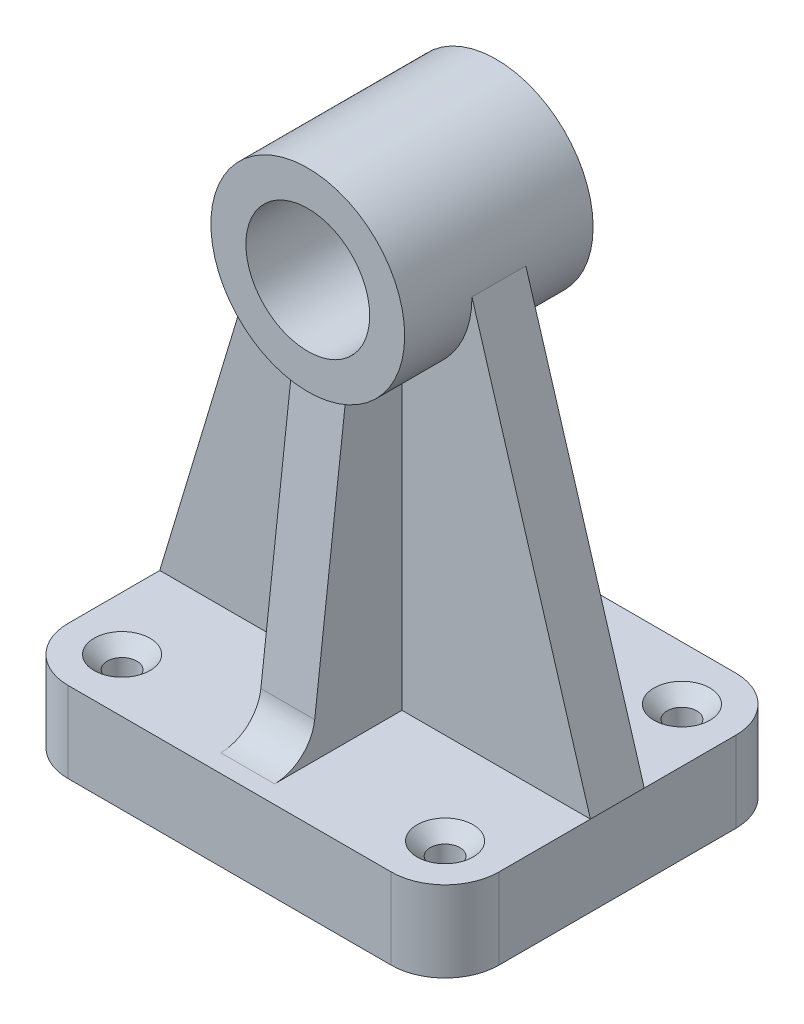
ISO-10303-21;
HEADER;
FILE_DESCRIPTION(('STEP AP214'),'2;1');
FILE_NAME('part.step','',(''),(''),'','','');
FILE_SCHEMA(('AUTOMOTIVE_DESIGN { 1 0 10303 214 1 1 1 1 }'));
ENDSEC;
DATA;
#1=APPLICATION_CONTEXT('core data for automotive mechanical design processes');
#2=APPLICATION_PROTOCOL_DEFINITION('international standard','automotive_design',2000,#1);
#3=PRODUCT_CONTEXT('',#1,'mechanical');
#4=PRODUCT('Part','Part','',(#3));
#5=PRODUCT_RELATED_PRODUCT_CATEGORY('part','',(#4));
#6=PRODUCT_DEFINITION_FORMATION('','',#4);
#7=PRODUCT_DEFINITION_CONTEXT('part definition',#1,'design');
#8=PRODUCT_DEFINITION('design','',#6,#7);
#9=PRODUCT_DEFINITION_SHAPE('','',#8);
#10=(LENGTH_UNIT() NAMED_UNIT(*) SI_UNIT(.MILLI.,.METRE.));
#11=(NAMED_UNIT(*) PLANE_ANGLE_UNIT() SI_UNIT($,.RADIAN.));
#12=(NAMED_UNIT(*) SI_UNIT($,.STERADIAN.) SOLID_ANGLE_UNIT());
#13=UNCERTAINTY_MEASURE_WITH_UNIT(LENGTH_MEASURE(1.E-05),#10,'distance_accuracy_value','');
#14=(GEOMETRIC_REPRESENTATION_CONTEXT(3) GLOBAL_UNCERTAINTY_ASSIGNED_CONTEXT((#13)) GLOBAL_UNIT_ASSIGNED_CONTEXT((#10,
#11,#12)) REPRESENTATION_CONTEXT('',''));
#15=CARTESIAN_POINT('',(0.,0.,0.));
#16=DIRECTION('',(0.,0.,1.));
#17=DIRECTION('',(1.,0.,0.));
#18=AXIS2_PLACEMENT_3D('',#15,#16,#17);
#19=CARTESIAN_POINT('',(0.,88.,5.));
#20=DIRECTION('',(0.,0.,1.));
#21=DIRECTION('',(1.,0.,0.));
#22=AXIS2_PLACEMENT_3D('',#19,#20,#21);
#23=PLANE('',#22);
#24=DIRECTION('',(1.,0.,0.));
#25=VECTOR('',#24,1.);
#26=CARTESIAN_POINT('',(-40.,15.,5.));
#27=LINE('',#26,#25);
#28=CARTESIAN_POINT('',(-40.,15.,5.));
#29=VERTEX_POINT('',#28);
#30=CARTESIAN_POINT('',(-5.,15.,5.));
#31=VERTEX_POINT('',#30);
#32=EDGE_CURVE('E209',#29,#31,#27,.T.);
#33=ORIENTED_EDGE('',*,*,#32,.T.);
#34=DIRECTION('',(0.,1.,0.));
#35=VECTOR('',#34,1.);
#36=CARTESIAN_POINT('',(-5.,88.,5.));
#37=LINE('',#36,#35);
#38=CARTESIAN_POINT('',(-5.,70.7083835342094,5.));
#39=VERTEX_POINT('',#38);
#40=EDGE_CURVE('E207',#31,#39,#37,.T.);
#41=ORIENTED_EDGE('',*,*,#40,.T.);
#42=CARTESIAN_POINT('',(0.,88.,5.));
#43=DIRECTION('',(0.,0.,-1.));
#44=DIRECTION('',(1.,0.,0.));
#45=AXIS2_PLACEMENT_3D('',#42,#43,#44);
#46=CIRCLE('',#45,18.);
#47=CARTESIAN_POINT('',(-18.,88.,5.));
#48=VERTEX_POINT('',#47);
#49=EDGE_CURVE('E195',#39,#48,#46,.T.);
#50=ORIENTED_EDGE('',*,*,#49,.T.);
#51=DIRECTION('',(-0.288550957217968,-0.95746453985962,0.));
#52=VECTOR('',#51,1.);
#53=CARTESIAN_POINT('',(-18.,88.,5.));
#54=LINE('',#53,#52);
#55=EDGE_CURVE('E305',#48,#29,#54,.T.);
#56=ORIENTED_EDGE('',*,*,#55,.T.);
#57=EDGE_LOOP('',(#33,#41,#50,#56));
#58=FACE_BOUND('',#57,.T.);
#59=ADVANCED_FACE('F44',(#58),#23,.T.);
#60=CARTESIAN_POINT('',(0.,88.,-5.));
#61=DIRECTION('',(0.,0.,1.));
#62=DIRECTION('',(1.,0.,0.));
#63=AXIS2_PLACEMENT_3D('',#60,#61,#62);
#64=PLANE('',#63);
#65=DIRECTION('',(0.,1.,0.));
#66=VECTOR('',#65,1.);
#67=CARTESIAN_POINT('',(-5.,88.,-5.));
#68=LINE('',#67,#66);
#69=CARTESIAN_POINT('',(-5.,15.,-5.));
#70=VERTEX_POINT('',#69);
#71=CARTESIAN_POINT('',(-5.,70.7083835342094,-5.));
#72=VERTEX_POINT('',#71);
#73=EDGE_CURVE('E238',#70,#72,#68,.T.);
#74=ORIENTED_EDGE('',*,*,#73,.F.);
#75=DIRECTION('',(1.,0.,0.));
#76=VECTOR('',#75,1.);
#77=CARTESIAN_POINT('',(-40.,15.,-5.));
#78=LINE('',#77,#76);
#79=CARTESIAN_POINT('',(-40.,15.,-5.));
#80=VERTEX_POINT('',#79);
#81=EDGE_CURVE('E320',#80,#70,#78,.T.);
#82=ORIENTED_EDGE('',*,*,#81,.F.);
#83=DIRECTION('',(-0.288550957217968,-0.95746453985962,0.));
#84=VECTOR('',#83,1.);
#85=CARTESIAN_POINT('',(-18.,88.,-5.));
#86=LINE('',#85,#84);
#87=CARTESIAN_POINT('',(-18.,88.,-5.));
#88=VERTEX_POINT('',#87);
#89=EDGE_CURVE('E311',#88,#80,#86,.T.);
#90=ORIENTED_EDGE('',*,*,#89,.F.);
#91=CARTESIAN_POINT('',(0.,88.,-5.));
#92=DIRECTION('',(0.,0.,-1.));
#93=DIRECTION('',(1.,0.,0.));
#94=AXIS2_PLACEMENT_3D('',#91,#92,#93);
#95=CIRCLE('',#94,18.);
#96=EDGE_CURVE('E296',#72,#88,#95,.T.);
#97=ORIENTED_EDGE('',*,*,#96,.F.);
#98=EDGE_LOOP('',(#74,#82,#90,#97));
#99=FACE_BOUND('',#98,.T.);
#100=ADVANCED_FACE('F429',(#99),#64,.F.);
#101=CARTESIAN_POINT('',(-30.,15.,22.));
#102=DIRECTION('',(0.,1.,0.));
#103=DIRECTION('',(0.,0.,1.));
#104=AXIS2_PLACEMENT_3D('',#101,#102,#103);
#105=PLANE('',#104);
#106=DIRECTION('',(-1.,0.,0.));
#107=VECTOR('',#106,1.);
#108=CARTESIAN_POINT('',(29.9999999999999,15.,-32.));
#109=LINE('',#108,#107);
#110=CARTESIAN_POINT('',(29.9999999999999,15.,-32.));
#111=VERTEX_POINT('',#110);
#112=CARTESIAN_POINT('',(-29.9999999999999,15.,-32.));
#113=VERTEX_POINT('',#112);
#114=EDGE_CURVE('E343',#111,#113,#109,.T.);
#115=ORIENTED_EDGE('',*,*,#114,.T.);
#116=CARTESIAN_POINT('',(-30.,15.,-22.));
#117=DIRECTION('',(0.,1.,0.));
#118=DIRECTION('',(0.,0.,1.));
#119=AXIS2_PLACEMENT_3D('',#116,#117,#118);
#120=CIRCLE('',#119,10.);
#121=CARTESIAN_POINT('',(-40.,15.,-21.9999999999999));
#122=VERTEX_POINT('',#121);
#123=EDGE_CURVE('E347',#113,#122,#120,.T.);
#124=ORIENTED_EDGE('',*,*,#123,.T.);
#125=DIRECTION('',(0.,0.,1.));
#126=VECTOR('',#125,1.);
#127=CARTESIAN_POINT('',(-40.,15.,-21.9999999999999));
#128=LINE('',#127,#126);
#129=EDGE_CURVE('E349',#122,#80,#128,.T.);
#130=ORIENTED_EDGE('',*,*,#129,.T.);
#131=ORIENTED_EDGE('',*,*,#81,.T.);
#132=DIRECTION('',(0.,0.,-1.));
#133=VECTOR('',#132,1.);
#134=CARTESIAN_POINT('',(-5.,15.,22.));
#135=LINE('',#134,#133);
#136=CARTESIAN_POINT('',(-5.,15.,-28.6658307795573));
#137=VERTEX_POINT('',#136);
#138=EDGE_CURVE('E245',#70,#137,#135,.T.);
#139=ORIENTED_EDGE('',*,*,#138,.T.);
#140=DIRECTION('',(1.,0.,0.));
#141=VECTOR('',#140,1.);
#142=CARTESIAN_POINT('',(5.,15.,-28.6658307795573));
#143=LINE('',#142,#141);
#144=CARTESIAN_POINT('',(5.,15.,-28.6658307795573));
#145=VERTEX_POINT('',#144);
#146=EDGE_CURVE('E393',#137,#145,#143,.T.);
#147=ORIENTED_EDGE('',*,*,#146,.T.);
#148=DIRECTION('',(0.,0.,-1.));
#149=VECTOR('',#148,1.);
#150=CARTESIAN_POINT('',(5.,15.,22.));
#151=LINE('',#150,#149);
#152=CARTESIAN_POINT('',(5.,15.,-5.));
#153=VERTEX_POINT('',#152);
#154=EDGE_CURVE('E248',#153,#145,#151,.T.);
#155=ORIENTED_EDGE('',*,*,#154,.F.);
#156=CARTESIAN_POINT('',(40.,15.,-5.));
#157=VERTEX_POINT('',#156);
#158=EDGE_CURVE('E316',#153,#157,#78,.T.);
#159=ORIENTED_EDGE('',*,*,#158,.T.);
#160=DIRECTION('',(0.,0.,-1.));
#161=VECTOR('',#160,1.);
#162=CARTESIAN_POINT('',(40.,15.,21.9999999999999));
#163=LINE('',#162,#161);
#164=CARTESIAN_POINT('',(40.,15.,-21.9999999999999));
#165=VERTEX_POINT('',#164);
#166=EDGE_CURVE('E340',#157,#165,#163,.T.);
#167=ORIENTED_EDGE('',*,*,#166,.T.);
#168=CARTESIAN_POINT('',(30.,15.,-22.));
#169=DIRECTION('',(0.,1.,0.));
#170=DIRECTION('',(0.,0.,1.));
#171=AXIS2_PLACEMENT_3D('',#168,#169,#170);
#172=CIRCLE('',#171,10.);
#173=EDGE_CURVE('E341',#165,#111,#172,.T.);
#174=ORIENTED_EDGE('',*,*,#173,.T.);
#175=EDGE_LOOP('',(#115,#124,#130,#131,#139,#147,#155,#159,#167,#174));
#176=FACE_BOUND('',#175,.T.);
#177=CARTESIAN_POINT('',(30.,15.,-22.));
#178=DIRECTION('',(0.,1.,0.));
#179=DIRECTION('',(0.,0.,1.));
#180=AXIS2_PLACEMENT_3D('',#177,#178,#179);
#181=CIRCLE('',#180,5.2);
#182=CARTESIAN_POINT('',(30.,15.,-16.8));
#183=VERTEX_POINT('',#182);
#184=EDGE_CURVE('E265',#183,#183,#181,.T.);
#185=ORIENTED_EDGE('',*,*,#184,.F.);
#186=EDGE_LOOP('',(#185));
#187=FACE_BOUND('',#186,.T.);
#188=CARTESIAN_POINT('',(-30.,15.,-22.));
#189=DIRECTION('',(0.,1.,0.));
#190=DIRECTION('',(0.,0.,1.));
#191=AXIS2_PLACEMENT_3D('',#188,#189,#190);
#192=CIRCLE('',#191,5.2);
#193=CARTESIAN_POINT('',(-30.,15.,-16.8));
#194=VERTEX_POINT('',#193);
#195=EDGE_CURVE('E251',#194,#194,#192,.T.);
#196=ORIENTED_EDGE('',*,*,#195,.F.);
#197=EDGE_LOOP('',(#196));
#198=FACE_BOUND('',#197,.T.);
#199=ADVANCED_FACE('F433',(#176,#187,#198),#105,.T.);
#200=CARTESIAN_POINT('',(-30.,15.,22.));
#201=DIRECTION('',(0.,-1.,0.));
#202=DIRECTION('',(0.,0.,-1.));
#203=AXIS2_PLACEMENT_3D('',#200,#201,#202);
#204=CYLINDRICAL_SURFACE('',#203,10.);
#205=CARTESIAN_POINT('',(-30.,0.,22.));
#206=DIRECTION('',(0.,1.,0.));
#207=DIRECTION('',(0.,0.,1.));
#208=AXIS2_PLACEMENT_3D('',#205,#206,#207);
#209=CIRCLE('',#208,10.);
#210=CARTESIAN_POINT('',(-40.,0.,21.9999999999999));
#211=VERTEX_POINT('',#210);
#212=CARTESIAN_POINT('',(-29.9999999999999,0.,32.));
#213=VERTEX_POINT('',#212);
#214=EDGE_CURVE('E328',#211,#213,#209,.T.);
#215=ORIENTED_EDGE('',*,*,#214,.T.);
#216=DIRECTION('',(0.,-1.,0.));
#217=VECTOR('',#216,1.);
#218=CARTESIAN_POINT('',(-29.9999999999999,15.,32.));
#219=LINE('',#218,#217);
#220=CARTESIAN_POINT('',(-29.9999999999999,15.,32.));
#221=VERTEX_POINT('',#220);
#222=EDGE_CURVE('E386',#221,#213,#219,.T.);
#223=ORIENTED_EDGE('',*,*,#222,.F.);
#224=CARTESIAN_POINT('',(-30.,15.,22.));
#225=DIRECTION('',(0.,1.,0.));
#226=DIRECTION('',(0.,0.,1.));
#227=AXIS2_PLACEMENT_3D('',#224,#225,#226);
#228=CIRCLE('',#227,10.);
#229=CARTESIAN_POINT('',(-40.,15.,21.9999999999999));
#230=VERTEX_POINT('',#229);
#231=EDGE_CURVE('E329',#230,#221,#228,.T.);
#232=ORIENTED_EDGE('',*,*,#231,.F.);
#233=DIRECTION('',(0.,-1.,0.));
#234=VECTOR('',#233,1.);
#235=CARTESIAN_POINT('',(-40.,15.,21.9999999999999));
#236=LINE('',#235,#234);
#237=EDGE_CURVE('E354',#230,#211,#236,.T.);
#238=ORIENTED_EDGE('',*,*,#237,.T.);
#239=EDGE_LOOP('',(#215,#223,#232,#238));
#240=FACE_BOUND('',#239,.T.);
#241=ADVANCED_FACE('F710',(#240),#204,.T.);
#242=CARTESIAN_POINT('',(-29.9999999999999,15.,32.));
#243=DIRECTION('',(0.,0.,-1.));
#244=DIRECTION('',(-1.,0.,0.));
#245=AXIS2_PLACEMENT_3D('',#242,#243,#244);
#246=PLANE('',#245);
#247=DIRECTION('',(0.,-1.,0.));
#248=VECTOR('',#247,1.);
#249=CARTESIAN_POINT('',(29.9999999999999,15.,32.));
#250=LINE('',#249,#248);
#251=CARTESIAN_POINT('',(29.9999999999999,15.,32.));
#252=VERTEX_POINT('',#251);
#253=CARTESIAN_POINT('',(29.9999999999999,0.,32.));
#254=VERTEX_POINT('',#253);
#255=EDGE_CURVE('E387',#252,#254,#250,.T.);
#256=ORIENTED_EDGE('',*,*,#255,.F.);
#257=DIRECTION('',(1.,0.,0.));
#258=VECTOR('',#257,1.);
#259=CARTESIAN_POINT('',(-29.9999999999999,15.,32.));
#260=LINE('',#259,#258);
#261=EDGE_CURVE('E334',#221,#252,#260,.T.);
#262=ORIENTED_EDGE('',*,*,#261,.F.);
#263=ORIENTED_EDGE('',*,*,#222,.T.);
#264=DIRECTION('',(1.,0.,0.));
#265=VECTOR('',#264,1.);
#266=CARTESIAN_POINT('',(-29.9999999999999,0.,32.));
#267=LINE('',#266,#265);
#268=EDGE_CURVE('E353',#213,#254,#267,.T.);
#269=ORIENTED_EDGE('',*,*,#268,.T.);
#270=EDGE_LOOP('',(#256,#262,#263,#269));
#271=FACE_BOUND('',#270,.T.);
#272=ADVANCED_FACE('F772',(#271),#246,.F.);
#273=CARTESIAN_POINT('',(30.,15.,22.));
#274=DIRECTION('',(0.,-1.,0.));
#275=DIRECTION('',(0.,0.,-1.));
#276=AXIS2_PLACEMENT_3D('',#273,#274,#275);
#277=CYLINDRICAL_SURFACE('',#276,10.);
#278=CARTESIAN_POINT('',(30.,0.,22.));
#279=DIRECTION('',(0.,1.,0.));
#280=DIRECTION('',(0.,0.,1.));
#281=AXIS2_PLACEMENT_3D('',#278,#279,#280);
#282=CIRCLE('',#281,10.);
#283=CARTESIAN_POINT('',(40.,0.,21.9999999999999));
#284=VERTEX_POINT('',#283);
#285=EDGE_CURVE('E356',#254,#284,#282,.T.);
#286=ORIENTED_EDGE('',*,*,#285,.T.);
#287=DIRECTION('',(0.,-1.,0.));
#288=VECTOR('',#287,1.);
#289=CARTESIAN_POINT('',(40.,15.,21.9999999999999));
#290=LINE('',#289,#288);
#291=CARTESIAN_POINT('',(40.,15.,21.9999999999999));
#292=VERTEX_POINT('',#291);
#293=EDGE_CURVE('E382',#292,#284,#290,.T.);
#294=ORIENTED_EDGE('',*,*,#293,.F.);
#295=CARTESIAN_POINT('',(30.,15.,22.));
#296=DIRECTION('',(0.,1.,0.));
#297=DIRECTION('',(0.,0.,1.));
#298=AXIS2_PLACEMENT_3D('',#295,#296,#297);
#299=CIRCLE('',#298,10.);
#300=EDGE_CURVE('E337',#252,#292,#299,.T.);
#301=ORIENTED_EDGE('',*,*,#300,.F.);
#302=ORIENTED_EDGE('',*,*,#255,.T.);
#303=EDGE_LOOP('',(#286,#294,#301,#302));
#304=FACE_BOUND('',#303,.T.);
#305=ADVANCED_FACE('F763',(#304),#277,.T.);
#306=CARTESIAN_POINT('',(40.,15.,0.));
#307=DIRECTION('',(-1.,0.,0.));
#308=DIRECTION('',(0.,0.,1.));
#309=AXIS2_PLACEMENT_3D('',#306,#307,#308);
#310=PLANE('',#309);
#311=DIRECTION('',(0.,0.,-1.));
#312=VECTOR('',#311,1.);
#313=CARTESIAN_POINT('',(40.,0.,0.));
#314=LINE('',#313,#312);
#315=CARTESIAN_POINT('',(40.,0.,-21.9999999999999));
#316=VERTEX_POINT('',#315);
#317=EDGE_CURVE('E357',#284,#316,#314,.T.);
#318=ORIENTED_EDGE('',*,*,#317,.T.);
#319=DIRECTION('',(0.,-1.,0.));
#320=VECTOR('',#319,1.);
#321=CARTESIAN_POINT('',(40.,15.,-21.9999999999999));
#322=LINE('',#321,#320);
#323=EDGE_CURVE('E379',#165,#316,#322,.T.);
#324=ORIENTED_EDGE('',*,*,#323,.F.);
#325=ORIENTED_EDGE('',*,*,#166,.F.);
#326=DIRECTION('',(0.,0.,-1.));
#327=VECTOR('',#326,1.);
#328=CARTESIAN_POINT('',(40.,15.,5.));
#329=LINE('',#328,#327);
#330=CARTESIAN_POINT('',(40.,15.,5.));
#331=VERTEX_POINT('',#330);
#332=EDGE_CURVE('E323',#331,#157,#329,.T.);
#333=ORIENTED_EDGE('',*,*,#332,.F.);
#334=EDGE_CURVE('E336',#292,#331,#163,.T.);
#335=ORIENTED_EDGE('',*,*,#334,.F.);
#336=ORIENTED_EDGE('',*,*,#293,.T.);
#337=EDGE_LOOP('',(#318,#324,#325,#333,#335,#336));
#338=FACE_BOUND('',#337,.T.);
#339=ADVANCED_FACE('F496',(#338),#310,.F.);
#340=CARTESIAN_POINT('',(30.,15.,-22.));
#341=DIRECTION('',(0.,-1.,0.));
#342=DIRECTION('',(0.,0.,-1.));
#343=AXIS2_PLACEMENT_3D('',#340,#341,#342);
#344=CYLINDRICAL_SURFACE('',#343,10.);
#345=CARTESIAN_POINT('',(30.,0.,-22.));
#346=DIRECTION('',(0.,1.,0.));
#347=DIRECTION('',(0.,0.,1.));
#348=AXIS2_PLACEMENT_3D('',#345,#346,#347);
#349=CIRCLE('',#348,10.);
#350=CARTESIAN_POINT('',(29.9999999999999,0.,-32.));
#351=VERTEX_POINT('',#350);
#352=EDGE_CURVE('E362',#316,#351,#349,.T.);
#353=ORIENTED_EDGE('',*,*,#352,.T.);
#354=DIRECTION('',(0.,-1.,0.));
#355=VECTOR('',#354,1.);
#356=CARTESIAN_POINT('',(29.9999999999999,15.,-32.));
#357=LINE('',#356,#355);
#358=EDGE_CURVE('E380',#111,#351,#357,.T.);
#359=ORIENTED_EDGE('',*,*,#358,.F.);
#360=ORIENTED_EDGE('',*,*,#173,.F.);
#361=ORIENTED_EDGE('',*,*,#323,.T.);
#362=EDGE_LOOP('',(#353,#359,#360,#361));
#363=FACE_BOUND('',#362,.T.);
#364=ADVANCED_FACE('F742',(#363),#344,.T.);
#365=CARTESIAN_POINT('',(29.9999999999999,15.,-32.));
#366=DIRECTION('',(0.,0.,1.));
#367=DIRECTION('',(1.,0.,0.));
#368=AXIS2_PLACEMENT_3D('',#365,#366,#367);
#369=PLANE('',#368);
#370=DIRECTION('',(-1.,0.,0.));
#371=VECTOR('',#370,1.);
#372=CARTESIAN_POINT('',(29.9999999999999,0.,-32.));
#373=LINE('',#372,#371);
#374=CARTESIAN_POINT('',(-29.9999999999999,0.,-32.));
#375=VERTEX_POINT('',#374);
#376=EDGE_CURVE('E365',#351,#375,#373,.T.);
#377=ORIENTED_EDGE('',*,*,#376,.T.);
#378=DIRECTION('',(0.,-1.,0.));
#379=VECTOR('',#378,1.);
#380=CARTESIAN_POINT('',(-29.9999999999999,15.,-32.));
#381=LINE('',#380,#379);
#382=EDGE_CURVE('E372',#113,#375,#381,.T.);
#383=ORIENTED_EDGE('',*,*,#382,.F.);
#384=ORIENTED_EDGE('',*,*,#114,.F.);
#385=ORIENTED_EDGE('',*,*,#358,.T.);
#386=EDGE_LOOP('',(#377,#383,#384,#385));
#387=FACE_BOUND('',#386,.T.);
#388=ADVANCED_FACE('F737',(#387),#369,.F.);
#389=CARTESIAN_POINT('',(-30.,15.,-22.));
#390=DIRECTION('',(0.,-1.,0.));
#391=DIRECTION('',(0.,0.,-1.));
#392=AXIS2_PLACEMENT_3D('',#389,#390,#391);
#393=CYLINDRICAL_SURFACE('',#392,10.);
#394=CARTESIAN_POINT('',(-30.,0.,-22.));
#395=DIRECTION('',(0.,1.,0.));
#396=DIRECTION('',(0.,0.,1.));
#397=AXIS2_PLACEMENT_3D('',#394,#395,#396);
#398=CIRCLE('',#397,10.);
#399=CARTESIAN_POINT('',(-40.,0.,-21.9999999999999));
#400=VERTEX_POINT('',#399);
#401=EDGE_CURVE('E368',#375,#400,#398,.T.);
#402=ORIENTED_EDGE('',*,*,#401,.T.);
#403=DIRECTION('',(0.,-1.,0.));
#404=VECTOR('',#403,1.);
#405=CARTESIAN_POINT('',(-40.,15.,-21.9999999999999));
#406=LINE('',#405,#404);
#407=EDGE_CURVE('E371',#122,#400,#406,.T.);
#408=ORIENTED_EDGE('',*,*,#407,.F.);
#409=ORIENTED_EDGE('',*,*,#123,.F.);
#410=ORIENTED_EDGE('',*,*,#382,.T.);
#411=EDGE_LOOP('',(#402,#408,#409,#410));
#412=FACE_BOUND('',#411,.T.);
#413=ADVANCED_FACE('F730',(#412),#393,.T.);
#414=CARTESIAN_POINT('',(-40.,15.,-21.9999999999999));
#415=DIRECTION('',(1.,0.,0.));
#416=DIRECTION('',(0.,0.,-1.));
#417=AXIS2_PLACEMENT_3D('',#414,#415,#416);
#418=PLANE('',#417);
#419=DIRECTION('',(0.,0.,1.));
#420=VECTOR('',#419,1.);
#421=CARTESIAN_POINT('',(-40.,0.,-21.9999999999999));
#422=LINE('',#421,#420);
#423=EDGE_CURVE('E331',#400,#211,#422,.T.);
#424=ORIENTED_EDGE('',*,*,#423,.T.);
#425=ORIENTED_EDGE('',*,*,#237,.F.);
#426=EDGE_CURVE('E346',#29,#230,#128,.T.);
#427=ORIENTED_EDGE('',*,*,#426,.F.);
#428=DIRECTION('',(0.,0.,-1.));
#429=VECTOR('',#428,1.);
#430=CARTESIAN_POINT('',(-40.,15.,5.));
#431=LINE('',#430,#429);
#432=EDGE_CURVE('E326',#29,#80,#431,.T.);
#433=ORIENTED_EDGE('',*,*,#432,.T.);
#434=ORIENTED_EDGE('',*,*,#129,.F.);
#435=ORIENTED_EDGE('',*,*,#407,.T.);
#436=EDGE_LOOP('',(#424,#425,#427,#433,#434,#435));
#437=FACE_BOUND('',#436,.T.);
#438=ADVANCED_FACE('F419',(#437),#418,.F.);
#439=DIRECTION('',(0.,0.,-1.));
#440=VECTOR('',#439,1.);
#441=CARTESIAN_POINT('',(5.,15.,22.));
#442=LINE('',#441,#440);
#443=CARTESIAN_POINT('',(5.,15.,28.6658307795573));
#444=VERTEX_POINT('',#443);
#445=CARTESIAN_POINT('',(5.,15.,5.));
#446=VERTEX_POINT('',#445);
#447=EDGE_CURVE('E58',#444,#446,#442,.T.);
#448=ORIENTED_EDGE('',*,*,#447,.F.);
#449=DIRECTION('',(1.,0.,0.));
#450=VECTOR('',#449,1.);
#451=CARTESIAN_POINT('',(-5.,15.,28.6658307795573));
#452=LINE('',#451,#450);
#453=CARTESIAN_POINT('',(-5.,15.,28.6658307795573));
#454=VERTEX_POINT('',#453);
#455=EDGE_CURVE('E407',#444,#454,#452,.F.);
#456=ORIENTED_EDGE('',*,*,#455,.T.);
#457=DIRECTION('',(0.,0.,-1.));
#458=VECTOR('',#457,1.);
#459=CARTESIAN_POINT('',(-5.,15.,22.));
#460=LINE('',#459,#458);
#461=EDGE_CURVE('E66',#454,#31,#460,.T.);
#462=ORIENTED_EDGE('',*,*,#461,.T.);
#463=ORIENTED_EDGE('',*,*,#32,.F.);
#464=ORIENTED_EDGE('',*,*,#426,.T.);
#465=ORIENTED_EDGE('',*,*,#231,.T.);
#466=ORIENTED_EDGE('',*,*,#261,.T.);
#467=ORIENTED_EDGE('',*,*,#300,.T.);
#468=ORIENTED_EDGE('',*,*,#334,.T.);
#469=EDGE_CURVE('E302',#446,#331,#27,.T.);
#470=ORIENTED_EDGE('',*,*,#469,.F.);
#471=EDGE_LOOP('',(#448,#456,#462,#463,#464,#465,#466,#467,#468,#470));
#472=FACE_BOUND('',#471,.T.);
#473=CARTESIAN_POINT('',(30.,15.,22.));
#474=DIRECTION('',(0.,1.,0.));
#475=DIRECTION('',(0.,0.,1.));
#476=AXIS2_PLACEMENT_3D('',#473,#474,#475);
#477=CIRCLE('',#476,5.2);
#478=CARTESIAN_POINT('',(30.,15.,27.2));
#479=VERTEX_POINT('',#478);
#480=EDGE_CURVE('E271',#479,#479,#477,.T.);
#481=ORIENTED_EDGE('',*,*,#480,.F.);
#482=EDGE_LOOP('',(#481));
#483=FACE_BOUND('',#482,.T.);
#484=CARTESIAN_POINT('',(-30.,15.,22.));
#485=DIRECTION('',(0.,1.,0.));
#486=DIRECTION('',(0.,0.,1.));
#487=AXIS2_PLACEMENT_3D('',#484,#485,#486);
#488=CIRCLE('',#487,5.2);
#489=CARTESIAN_POINT('',(-30.,15.,27.2));
#490=VERTEX_POINT('',#489);
#491=EDGE_CURVE('E278',#490,#490,#488,.T.);
#492=ORIENTED_EDGE('',*,*,#491,.F.);
#493=EDGE_LOOP('',(#492));
#494=FACE_BOUND('',#493,.T.);
#495=ADVANCED_FACE('F412',(#472,#483,#494),#105,.T.);
#496=CARTESIAN_POINT('',(-30.,0.,22.));
#497=DIRECTION('',(0.,1.,0.));
#498=DIRECTION('',(0.,0.,1.));
#499=AXIS2_PLACEMENT_3D('',#496,#497,#498);
#500=PLANE('',#499);
#501=ORIENTED_EDGE('',*,*,#401,.F.);
#502=ORIENTED_EDGE('',*,*,#376,.F.);
#503=ORIENTED_EDGE('',*,*,#352,.F.);
#504=ORIENTED_EDGE('',*,*,#317,.F.);
#505=ORIENTED_EDGE('',*,*,#285,.F.);
#506=ORIENTED_EDGE('',*,*,#268,.F.);
#507=ORIENTED_EDGE('',*,*,#214,.F.);
#508=ORIENTED_EDGE('',*,*,#423,.F.);
#509=EDGE_LOOP('',(#501,#502,#503,#504,#505,#506,#507,#508));
#510=FACE_BOUND('',#509,.T.);
#511=CARTESIAN_POINT('',(-30.,0.,-22.));
#512=DIRECTION('',(0.,1.,0.));
#513=DIRECTION('',(0.,0.,1.));
#514=AXIS2_PLACEMENT_3D('',#511,#512,#513);
#515=CIRCLE('',#514,2.75);
#516=CARTESIAN_POINT('',(-30.,0.,-19.25));
#517=VERTEX_POINT('',#516);
#518=EDGE_CURVE('E259',#517,#517,#515,.T.);
#519=ORIENTED_EDGE('',*,*,#518,.T.);
#520=EDGE_LOOP('',(#519));
#521=FACE_BOUND('',#520,.T.);
#522=CARTESIAN_POINT('',(30.,0.,-22.));
#523=DIRECTION('',(0.,1.,0.));
#524=DIRECTION('',(0.,0.,1.));
#525=AXIS2_PLACEMENT_3D('',#522,#523,#524);
#526=CIRCLE('',#525,2.75);
#527=CARTESIAN_POINT('',(30.,0.,-19.25));
#528=VERTEX_POINT('',#527);
#529=EDGE_CURVE('E268',#528,#528,#526,.T.);
#530=ORIENTED_EDGE('',*,*,#529,.T.);
#531=EDGE_LOOP('',(#530));
#532=FACE_BOUND('',#531,.T.);
#533=CARTESIAN_POINT('',(30.,0.,22.));
#534=DIRECTION('',(0.,1.,0.));
#535=DIRECTION('',(0.,0.,1.));
#536=AXIS2_PLACEMENT_3D('',#533,#534,#535);
#537=CIRCLE('',#536,2.75);
#538=CARTESIAN_POINT('',(30.,0.,24.75));
#539=VERTEX_POINT('',#538);
#540=EDGE_CURVE('E280',#539,#539,#537,.T.);
#541=ORIENTED_EDGE('',*,*,#540,.T.);
#542=EDGE_LOOP('',(#541));
#543=FACE_BOUND('',#542,.T.);
#544=CARTESIAN_POINT('',(-30.,0.,22.));
#545=DIRECTION('',(0.,1.,0.));
#546=DIRECTION('',(0.,0.,1.));
#547=AXIS2_PLACEMENT_3D('',#544,#545,#546);
#548=CIRCLE('',#547,2.75);
#549=CARTESIAN_POINT('',(-30.,0.,24.75));
#550=VERTEX_POINT('',#549);
#551=EDGE_CURVE('E289',#550,#550,#548,.T.);
#552=ORIENTED_EDGE('',*,*,#551,.T.);
#553=EDGE_LOOP('',(#552));
#554=FACE_BOUND('',#553,.T.);
#555=ADVANCED_FACE('F663',(#510,#521,#532,#543,#554),#500,.F.);
#556=CARTESIAN_POINT('',(-18.,88.,5.));
#557=DIRECTION('',(0.95746453985962,-0.288550957217968,0.));
#558=DIRECTION('',(0.288550957217968,0.95746453985962,0.));
#559=AXIS2_PLACEMENT_3D('',#556,#557,#558);
#560=PLANE('',#559);
#561=ORIENTED_EDGE('',*,*,#89,.T.);
#562=ORIENTED_EDGE('',*,*,#432,.F.);
#563=ORIENTED_EDGE('',*,*,#55,.F.);
#564=DIRECTION('',(0.,0.,-1.));
#565=VECTOR('',#564,1.);
#566=CARTESIAN_POINT('',(-18.,88.,5.));
#567=LINE('',#566,#565);
#568=EDGE_CURVE('E203',#48,#88,#567,.T.);
#569=ORIENTED_EDGE('',*,*,#568,.T.);
#570=EDGE_LOOP('',(#561,#562,#563,#569));
#571=FACE_BOUND('',#570,.T.);
#572=ADVANCED_FACE('F422',(#571),#560,.F.);
#573=CARTESIAN_POINT('',(18.,88.,5.));
#574=DIRECTION('',(-0.95746453985962,-0.288550957217968,0.));
#575=DIRECTION('',(0.288550957217968,-0.95746453985962,0.));
#576=AXIS2_PLACEMENT_3D('',#573,#574,#575);
#577=PLANE('',#576);
#578=DIRECTION('',(-0.288550957217968,0.95746453985962,0.));
#579=VECTOR('',#578,1.);
#580=CARTESIAN_POINT('',(18.,88.,-5.));
#581=LINE('',#580,#579);
#582=CARTESIAN_POINT('',(18.,88.,-5.));
#583=VERTEX_POINT('',#582);
#584=EDGE_CURVE('E206',#157,#583,#581,.T.);
#585=ORIENTED_EDGE('',*,*,#584,.T.);
#586=DIRECTION('',(0.,0.,-1.));
#587=VECTOR('',#586,1.);
#588=CARTESIAN_POINT('',(18.,88.,5.));
#589=LINE('',#588,#587);
#590=CARTESIAN_POINT('',(18.,88.,5.));
#591=VERTEX_POINT('',#590);
#592=EDGE_CURVE('E310',#591,#583,#589,.T.);
#593=ORIENTED_EDGE('',*,*,#592,.F.);
#594=DIRECTION('',(-0.288550957217968,0.95746453985962,0.));
#595=VECTOR('',#594,1.);
#596=CARTESIAN_POINT('',(18.,88.,5.));
#597=LINE('',#596,#595);
#598=EDGE_CURVE('E307',#331,#591,#597,.T.);
#599=ORIENTED_EDGE('',*,*,#598,.F.);
#600=ORIENTED_EDGE('',*,*,#332,.T.);
#601=EDGE_LOOP('',(#585,#593,#599,#600));
#602=FACE_BOUND('',#601,.T.);
#603=ADVANCED_FACE('F481',(#602),#577,.F.);
#604=DIRECTION('',(0.,1.,0.));
#605=VECTOR('',#604,1.);
#606=CARTESIAN_POINT('',(5.,88.,5.));
#607=LINE('',#606,#605);
#608=CARTESIAN_POINT('',(5.,70.7083835342094,5.));
#609=VERTEX_POINT('',#608);
#610=EDGE_CURVE('E223',#446,#609,#607,.T.);
#611=ORIENTED_EDGE('',*,*,#610,.F.);
#612=ORIENTED_EDGE('',*,*,#469,.T.);
#613=ORIENTED_EDGE('',*,*,#598,.T.);
#614=EDGE_CURVE('E202',#591,#609,#46,.T.);
#615=ORIENTED_EDGE('',*,*,#614,.T.);
#616=EDGE_LOOP('',(#611,#612,#613,#615));
#617=FACE_BOUND('',#616,.T.);
#618=ADVANCED_FACE('F472',(#617),#23,.T.);
#619=ORIENTED_EDGE('',*,*,#158,.F.);
#620=DIRECTION('',(0.,1.,0.));
#621=VECTOR('',#620,1.);
#622=CARTESIAN_POINT('',(5.,88.,-5.));
#623=LINE('',#622,#621);
#624=CARTESIAN_POINT('',(5.,70.7083835342094,-5.));
#625=VERTEX_POINT('',#624);
#626=EDGE_CURVE('E246',#153,#625,#623,.T.);
#627=ORIENTED_EDGE('',*,*,#626,.T.);
#628=EDGE_CURVE('E309',#583,#625,#95,.T.);
#629=ORIENTED_EDGE('',*,*,#628,.F.);
#630=ORIENTED_EDGE('',*,*,#584,.F.);
#631=EDGE_LOOP('',(#619,#627,#629,#630));
#632=FACE_BOUND('',#631,.T.);
#633=ADVANCED_FACE('F446',(#632),#64,.F.);
#634=CARTESIAN_POINT('',(0.,88.,17.5));
#635=DIRECTION('',(0.,0.,1.));
#636=DIRECTION('',(1.,0.,0.));
#637=AXIS2_PLACEMENT_3D('',#634,#635,#636);
#638=PLANE('',#637);
#639=CARTESIAN_POINT('',(0.,88.,17.5));
#640=DIRECTION('',(0.,0.,1.));
#641=DIRECTION('',(1.,0.,0.));
#642=AXIS2_PLACEMENT_3D('',#639,#640,#641);
#643=CIRCLE('',#642,11.5);
#644=CARTESIAN_POINT('',(11.5,88.,17.5));
#645=VERTEX_POINT('',#644);
#646=EDGE_CURVE('E287',#645,#645,#643,.T.);
#647=ORIENTED_EDGE('',*,*,#646,.F.);
#648=EDGE_LOOP('',(#647));
#649=FACE_BOUND('',#648,.T.);
#650=CARTESIAN_POINT('',(0.,88.,17.5));
#651=DIRECTION('',(0.,0.,1.));
#652=DIRECTION('',(1.,0.,0.));
#653=AXIS2_PLACEMENT_3D('',#650,#651,#652);
#654=CIRCLE('',#653,18.);
#655=CARTESIAN_POINT('',(18.,88.,17.5));
#656=VERTEX_POINT('',#655);
#657=EDGE_CURVE('E297',#656,#656,#654,.T.);
#658=ORIENTED_EDGE('',*,*,#657,.T.);
#659=EDGE_LOOP('',(#658));
#660=FACE_BOUND('',#659,.T.);
#661=ADVANCED_FACE('F488',(#649,#660),#638,.T.);
#662=CARTESIAN_POINT('',(0.,88.,-17.5));
#663=DIRECTION('',(0.,0.,1.));
#664=DIRECTION('',(1.,0.,0.));
#665=AXIS2_PLACEMENT_3D('',#662,#663,#664);
#666=PLANE('',#665);
#667=CARTESIAN_POINT('',(0.,88.,-17.5));
#668=DIRECTION('',(0.,0.,1.));
#669=DIRECTION('',(1.,0.,0.));
#670=AXIS2_PLACEMENT_3D('',#667,#668,#669);
#671=CIRCLE('',#670,11.5);
#672=CARTESIAN_POINT('',(11.5,88.,-17.5));
#673=VERTEX_POINT('',#672);
#674=EDGE_CURVE('E288',#673,#673,#671,.T.);
#675=ORIENTED_EDGE('',*,*,#674,.T.);
#676=EDGE_LOOP('',(#675));
#677=FACE_BOUND('',#676,.T.);
#678=CARTESIAN_POINT('',(0.,88.,-17.5));
#679=DIRECTION('',(0.,0.,1.));
#680=DIRECTION('',(1.,0.,0.));
#681=AXIS2_PLACEMENT_3D('',#678,#679,#680);
#682=CIRCLE('',#681,18.);
#683=CARTESIAN_POINT('',(18.,88.,-17.5));
#684=VERTEX_POINT('',#683);
#685=EDGE_CURVE('E291',#684,#684,#682,.T.);
#686=ORIENTED_EDGE('',*,*,#685,.F.);
#687=EDGE_LOOP('',(#686));
#688=FACE_BOUND('',#687,.T.);
#689=ADVANCED_FACE('F685',(#677,#688),#666,.F.);
#690=CARTESIAN_POINT('',(0.,88.,17.5));
#691=DIRECTION('',(0.,0.,-1.));
#692=DIRECTION('',(-1.,0.,0.));
#693=AXIS2_PLACEMENT_3D('',#690,#691,#692);
#694=CYLINDRICAL_SURFACE('',#693,18.);
#695=ORIENTED_EDGE('',*,*,#685,.T.);
#696=EDGE_LOOP('',(#695));
#697=FACE_BOUND('',#696,.T.);
#698=DIRECTION('',(0.,0.,-1.));
#699=VECTOR('',#698,1.);
#700=CARTESIAN_POINT('',(5.,70.7083835342094,17.5));
#701=LINE('',#700,#699);
#702=CARTESIAN_POINT('',(5.,70.7083835342094,-15.4162819459571));
#703=VERTEX_POINT('',#702);
#704=EDGE_CURVE('E243',#625,#703,#701,.T.);
#705=ORIENTED_EDGE('',*,*,#704,.T.);
#706=CARTESIAN_POINT('',(0.,88.,-13.3727272727273));
#707=DIRECTION('',(0.,-0.117365044853064,0.993088841064403));
#708=DIRECTION('',(0.,-0.993088841064403,-0.117365044853064));
#709=AXIS2_PLACEMENT_3D('',#706,#707,#708);
#710=ELLIPSE('',#709,18.1252665982103,18.);
#711=CARTESIAN_POINT('',(-5.,70.7083835342094,-15.4162819459571));
#712=VERTEX_POINT('',#711);
#713=EDGE_CURVE('E253',#703,#712,#710,.F.);
#714=ORIENTED_EDGE('',*,*,#713,.T.);
#715=DIRECTION('',(0.,0.,-1.));
#716=VECTOR('',#715,1.);
#717=CARTESIAN_POINT('',(-5.,70.7083835342094,17.5));
#718=LINE('',#717,#716);
#719=EDGE_CURVE('E232',#72,#712,#718,.T.);
#720=ORIENTED_EDGE('',*,*,#719,.F.);
#721=ORIENTED_EDGE('',*,*,#96,.T.);
#722=ORIENTED_EDGE('',*,*,#568,.F.);
#723=ORIENTED_EDGE('',*,*,#49,.F.);
#724=DIRECTION('',(0.,0.,-1.));
#725=VECTOR('',#724,1.);
#726=CARTESIAN_POINT('',(-5.,70.7083835342094,17.5));
#727=LINE('',#726,#725);
#728=CARTESIAN_POINT('',(-5.,70.7083835342094,15.4162819459571));
#729=VERTEX_POINT('',#728);
#730=EDGE_CURVE('E196',#729,#39,#727,.T.);
#731=ORIENTED_EDGE('',*,*,#730,.F.);
#732=CARTESIAN_POINT('',(0.,88.,13.3727272727273));
#733=DIRECTION('',(0.,0.117365044853064,0.993088841064403));
#734=DIRECTION('',(0.,0.993088841064403,-0.117365044853064));
#735=AXIS2_PLACEMENT_3D('',#732,#733,#734);
#736=ELLIPSE('',#735,18.1252665982103,18.);
#737=CARTESIAN_POINT('',(5.,70.7083835342094,15.4162819459571));
#738=VERTEX_POINT('',#737);
#739=EDGE_CURVE('E226',#729,#738,#736,.T.);
#740=ORIENTED_EDGE('',*,*,#739,.T.);
#741=DIRECTION('',(0.,0.,-1.));
#742=VECTOR('',#741,1.);
#743=CARTESIAN_POINT('',(5.,70.7083835342094,17.5));
#744=LINE('',#743,#742);
#745=EDGE_CURVE('E224',#738,#609,#744,.T.);
#746=ORIENTED_EDGE('',*,*,#745,.T.);
#747=ORIENTED_EDGE('',*,*,#614,.F.);
#748=ORIENTED_EDGE('',*,*,#592,.T.);
#749=ORIENTED_EDGE('',*,*,#628,.T.);
#750=EDGE_LOOP('',(#705,#714,#720,#721,#722,#723,#731,#740,#746,#747,#748,#749));
#751=FACE_BOUND('',#750,.T.);
#752=ORIENTED_EDGE('',*,*,#657,.F.);
#753=EDGE_LOOP('',(#752));
#754=FACE_BOUND('',#753,.T.);
#755=ADVANCED_FACE('F192',(#697,#751,#754),#694,.T.);
#756=CARTESIAN_POINT('',(0.,88.,17.5));
#757=DIRECTION('',(0.,0.,-1.));
#758=DIRECTION('',(-1.,0.,0.));
#759=AXIS2_PLACEMENT_3D('',#756,#757,#758);
#760=CYLINDRICAL_SURFACE('',#759,11.5);
#761=ORIENTED_EDGE('',*,*,#674,.F.);
#762=EDGE_LOOP('',(#761));
#763=FACE_BOUND('',#762,.T.);
#764=ORIENTED_EDGE('',*,*,#646,.T.);
#765=EDGE_LOOP('',(#764));
#766=FACE_BOUND('',#765,.T.);
#767=ADVANCED_FACE('F643',(#763,#766),#760,.F.);
#768=CARTESIAN_POINT('',(-30.,15.,22.));
#769=DIRECTION('',(0.,1.,0.));
#770=DIRECTION('',(0.,0.,1.));
#771=AXIS2_PLACEMENT_3D('',#768,#769,#770);
#772=CYLINDRICAL_SURFACE('',#771,2.75);
#773=ORIENTED_EDGE('',*,*,#551,.F.);
#774=EDGE_LOOP('',(#773));
#775=FACE_BOUND('',#774,.T.);
#776=CARTESIAN_POINT('',(-30.,12.55,22.));
#777=DIRECTION('',(0.,1.,0.));
#778=DIRECTION('',(0.,0.,1.));
#779=AXIS2_PLACEMENT_3D('',#776,#777,#778);
#780=CIRCLE('',#779,2.75);
#781=CARTESIAN_POINT('',(-30.,12.55,24.75));
#782=VERTEX_POINT('',#781);
#783=EDGE_CURVE('E285',#782,#782,#780,.T.);
#784=ORIENTED_EDGE('',*,*,#783,.T.);
#785=EDGE_LOOP('',(#784));
#786=FACE_BOUND('',#785,.T.);
#787=ADVANCED_FACE('F634',(#775,#786),#772,.F.);
#788=CARTESIAN_POINT('',(-30.,15.,22.));
#789=DIRECTION('',(0.,1.,0.));
#790=DIRECTION('',(0.,0.,1.));
#791=AXIS2_PLACEMENT_3D('',#788,#789,#790);
#792=CONICAL_SURFACE('',#791,5.2,0.785398163397448);
#793=ORIENTED_EDGE('',*,*,#783,.F.);
#794=EDGE_LOOP('',(#793));
#795=FACE_BOUND('',#794,.T.);
#796=ORIENTED_EDGE('',*,*,#491,.T.);
#797=EDGE_LOOP('',(#796));
#798=FACE_BOUND('',#797,.T.);
#799=ADVANCED_FACE('F622',(#795,#798),#792,.F.);
#800=CARTESIAN_POINT('',(30.,15.,22.));
#801=DIRECTION('',(0.,1.,0.));
#802=DIRECTION('',(0.,0.,1.));
#803=AXIS2_PLACEMENT_3D('',#800,#801,#802);
#804=CYLINDRICAL_SURFACE('',#803,2.75);
#805=ORIENTED_EDGE('',*,*,#540,.F.);
#806=EDGE_LOOP('',(#805));
#807=FACE_BOUND('',#806,.T.);
#808=CARTESIAN_POINT('',(30.,12.55,22.));
#809=DIRECTION('',(0.,1.,0.));
#810=DIRECTION('',(0.,0.,1.));
#811=AXIS2_PLACEMENT_3D('',#808,#809,#810);
#812=CIRCLE('',#811,2.75);
#813=CARTESIAN_POINT('',(30.,12.55,24.75));
#814=VERTEX_POINT('',#813);
#815=EDGE_CURVE('E273',#814,#814,#812,.T.);
#816=ORIENTED_EDGE('',*,*,#815,.T.);
#817=EDGE_LOOP('',(#816));
#818=FACE_BOUND('',#817,.T.);
#819=ADVANCED_FACE('F612',(#807,#818),#804,.F.);
#820=CARTESIAN_POINT('',(30.,15.,22.));
#821=DIRECTION('',(0.,1.,0.));
#822=DIRECTION('',(0.,0.,1.));
#823=AXIS2_PLACEMENT_3D('',#820,#821,#822);
#824=CONICAL_SURFACE('',#823,5.2,0.785398163397448);
#825=ORIENTED_EDGE('',*,*,#815,.F.);
#826=EDGE_LOOP('',(#825));
#827=FACE_BOUND('',#826,.T.);
#828=ORIENTED_EDGE('',*,*,#480,.T.);
#829=EDGE_LOOP('',(#828));
#830=FACE_BOUND('',#829,.T.);
#831=ADVANCED_FACE('F601',(#827,#830),#824,.F.);
#832=CARTESIAN_POINT('',(30.,15.,-22.));
#833=DIRECTION('',(0.,1.,0.));
#834=DIRECTION('',(0.,0.,1.));
#835=AXIS2_PLACEMENT_3D('',#832,#833,#834);
#836=CYLINDRICAL_SURFACE('',#835,2.75);
#837=ORIENTED_EDGE('',*,*,#529,.F.);
#838=EDGE_LOOP('',(#837));
#839=FACE_BOUND('',#838,.T.);
#840=CARTESIAN_POINT('',(30.,12.55,-22.));
#841=DIRECTION('',(0.,1.,0.));
#842=DIRECTION('',(0.,0.,1.));
#843=AXIS2_PLACEMENT_3D('',#840,#841,#842);
#844=CIRCLE('',#843,2.75);
#845=CARTESIAN_POINT('',(30.,12.55,-19.25));
#846=VERTEX_POINT('',#845);
#847=EDGE_CURVE('E264',#846,#846,#844,.T.);
#848=ORIENTED_EDGE('',*,*,#847,.T.);
#849=EDGE_LOOP('',(#848));
#850=FACE_BOUND('',#849,.T.);
#851=ADVANCED_FACE('F591',(#839,#850),#836,.F.);
#852=CARTESIAN_POINT('',(30.,15.,-22.));
#853=DIRECTION('',(0.,1.,0.));
#854=DIRECTION('',(0.,0.,1.));
#855=AXIS2_PLACEMENT_3D('',#852,#853,#854);
#856=CONICAL_SURFACE('',#855,5.2,0.785398163397448);
#857=ORIENTED_EDGE('',*,*,#847,.F.);
#858=EDGE_LOOP('',(#857));
#859=FACE_BOUND('',#858,.T.);
#860=ORIENTED_EDGE('',*,*,#184,.T.);
#861=EDGE_LOOP('',(#860));
#862=FACE_BOUND('',#861,.T.);
#863=ADVANCED_FACE('F583',(#859,#862),#856,.F.);
#864=CARTESIAN_POINT('',(-30.,15.,-22.));
#865=DIRECTION('',(0.,1.,0.));
#866=DIRECTION('',(0.,0.,1.));
#867=AXIS2_PLACEMENT_3D('',#864,#865,#866);
#868=CYLINDRICAL_SURFACE('',#867,2.75);
#869=ORIENTED_EDGE('',*,*,#518,.F.);
#870=EDGE_LOOP('',(#869));
#871=FACE_BOUND('',#870,.T.);
#872=CARTESIAN_POINT('',(-30.,12.55,-22.));
#873=DIRECTION('',(0.,1.,0.));
#874=DIRECTION('',(0.,0.,1.));
#875=AXIS2_PLACEMENT_3D('',#872,#873,#874);
#876=CIRCLE('',#875,2.75);
#877=CARTESIAN_POINT('',(-30.,12.55,-19.25));
#878=VERTEX_POINT('',#877);
#879=EDGE_CURVE('E258',#878,#878,#876,.T.);
#880=ORIENTED_EDGE('',*,*,#879,.T.);
#881=EDGE_LOOP('',(#880));
#882=FACE_BOUND('',#881,.T.);
#883=ADVANCED_FACE('F469',(#871,#882),#868,.F.);
#884=CARTESIAN_POINT('',(-30.,15.,-22.));
#885=DIRECTION('',(0.,1.,0.));
#886=DIRECTION('',(0.,0.,1.));
#887=AXIS2_PLACEMENT_3D('',#884,#885,#886);
#888=CONICAL_SURFACE('',#887,5.2,0.785398163397448);
#889=ORIENTED_EDGE('',*,*,#879,.F.);
#890=EDGE_LOOP('',(#889));
#891=FACE_BOUND('',#890,.T.);
#892=ORIENTED_EDGE('',*,*,#195,.T.);
#893=EDGE_LOOP('',(#892));
#894=FACE_BOUND('',#893,.T.);
#895=ADVANCED_FACE('F456',(#891,#894),#888,.F.);
#896=CARTESIAN_POINT('',(0.,70.,-15.5));
#897=DIRECTION('',(0.,-0.117365044853064,0.993088841064403));
#898=DIRECTION('',(0.,-0.993088841064403,-0.117365044853064));
#899=AXIS2_PLACEMENT_3D('',#896,#897,#898);
#900=PLANE('',#899);
#901=DIRECTION('',(0.,-0.993088841064403,-0.117365044853064));
#902=VECTOR('',#901,1.);
#903=CARTESIAN_POINT('',(5.,70.,-15.5));
#904=LINE('',#903,#902);
#905=CARTESIAN_POINT('',(5.,21.619762163602,-21.2176644715742));
#906=VERTEX_POINT('',#905);
#907=EDGE_CURVE('E231',#703,#906,#904,.T.);
#908=ORIENTED_EDGE('',*,*,#907,.T.);
#909=DIRECTION('',(-1.,0.,0.));
#910=VECTOR('',#909,1.);
#911=CARTESIAN_POINT('',(-5.,21.619762163602,-21.2176644715742));
#912=LINE('',#911,#910);
#913=CARTESIAN_POINT('',(-5.,21.619762163602,-21.2176644715742));
#914=VERTEX_POINT('',#913);
#915=EDGE_CURVE('E394',#906,#914,#912,.T.);
#916=ORIENTED_EDGE('',*,*,#915,.T.);
#917=DIRECTION('',(0.,-0.993088841064403,-0.117365044853064));
#918=VECTOR('',#917,1.);
#919=CARTESIAN_POINT('',(-5.,70.,-15.5));
#920=LINE('',#919,#918);
#921=EDGE_CURVE('E234',#712,#914,#920,.T.);
#922=ORIENTED_EDGE('',*,*,#921,.F.);
#923=ORIENTED_EDGE('',*,*,#713,.F.);
#924=EDGE_LOOP('',(#908,#916,#922,#923));
#925=FACE_BOUND('',#924,.T.);
#926=ADVANCED_FACE('F457',(#925),#900,.F.);
#927=CARTESIAN_POINT('',(5.,53.,0.));
#928=DIRECTION('',(1.,0.,0.));
#929=DIRECTION('',(0.,0.,-1.));
#930=AXIS2_PLACEMENT_3D('',#927,#928,#929);
#931=PLANE('',#930);
#932=ORIENTED_EDGE('',*,*,#626,.F.);
#933=ORIENTED_EDGE('',*,*,#154,.T.);
#934=CARTESIAN_POINT('',(5.,22.5,-28.6658307795573));
#935=DIRECTION('',(1.,0.,0.));
#936=DIRECTION('',(0.,0.,-1.));
#937=AXIS2_PLACEMENT_3D('',#934,#935,#936);
#938=CIRCLE('',#937,7.5);
#939=EDGE_CURVE('E402',#145,#906,#938,.F.);
#940=ORIENTED_EDGE('',*,*,#939,.T.);
#941=ORIENTED_EDGE('',*,*,#907,.F.);
#942=ORIENTED_EDGE('',*,*,#704,.F.);
#943=EDGE_LOOP('',(#932,#933,#940,#941,#942));
#944=FACE_BOUND('',#943,.T.);
#945=ADVANCED_FACE('F451',(#944),#931,.T.);
#946=CARTESIAN_POINT('',(-5.,53.,0.));
#947=DIRECTION('',(1.,0.,0.));
#948=DIRECTION('',(0.,0.,-1.));
#949=AXIS2_PLACEMENT_3D('',#946,#947,#948);
#950=PLANE('',#949);
#951=ORIENTED_EDGE('',*,*,#138,.F.);
#952=ORIENTED_EDGE('',*,*,#73,.T.);
#953=ORIENTED_EDGE('',*,*,#719,.T.);
#954=ORIENTED_EDGE('',*,*,#921,.T.);
#955=CARTESIAN_POINT('',(-5.,22.5,-28.6658307795573));
#956=DIRECTION('',(1.,0.,0.));
#957=DIRECTION('',(0.,0.,-1.));
#958=AXIS2_PLACEMENT_3D('',#955,#956,#957);
#959=CIRCLE('',#958,7.5);
#960=EDGE_CURVE('E400',#914,#137,#959,.T.);
#961=ORIENTED_EDGE('',*,*,#960,.T.);
#962=EDGE_LOOP('',(#951,#952,#953,#954,#961));
#963=FACE_BOUND('',#962,.T.);
#964=ADVANCED_FACE('F436',(#963),#950,.F.);
#965=CARTESIAN_POINT('',(0.,22.5,-28.6658307795573));
#966=DIRECTION('',(-1.,0.,0.));
#967=DIRECTION('',(0.,0.,1.));
#968=AXIS2_PLACEMENT_3D('',#965,#966,#967);
#969=CYLINDRICAL_SURFACE('',#968,7.5);
#970=ORIENTED_EDGE('',*,*,#939,.F.);
#971=ORIENTED_EDGE('',*,*,#146,.F.);
#972=ORIENTED_EDGE('',*,*,#960,.F.);
#973=ORIENTED_EDGE('',*,*,#915,.F.);
#974=EDGE_LOOP('',(#970,#971,#972,#973));
#975=FACE_BOUND('',#974,.T.);
#976=ADVANCED_FACE('F445',(#975),#969,.F.);
#977=CARTESIAN_POINT('',(0.,70.,15.5));
#978=DIRECTION('',(0.,0.117365044853064,0.993088841064403));
#979=DIRECTION('',(0.,-0.993088841064403,0.117365044853064));
#980=AXIS2_PLACEMENT_3D('',#977,#978,#979);
#981=PLANE('',#980);
#982=DIRECTION('',(0.,-0.993088841064403,0.117365044853064));
#983=VECTOR('',#982,1.);
#984=CARTESIAN_POINT('',(-5.,70.,15.5));
#985=LINE('',#984,#983);
#986=CARTESIAN_POINT('',(-5.,21.619762163602,21.2176644715742));
#987=VERTEX_POINT('',#986);
#988=EDGE_CURVE('E214',#729,#987,#985,.T.);
#989=ORIENTED_EDGE('',*,*,#988,.T.);
#990=DIRECTION('',(1.,0.,0.));
#991=VECTOR('',#990,1.);
#992=CARTESIAN_POINT('',(5.,21.619762163602,21.2176644715742));
#993=LINE('',#992,#991);
#994=CARTESIAN_POINT('',(5.,21.619762163602,21.2176644715742));
#995=VERTEX_POINT('',#994);
#996=EDGE_CURVE('E401',#987,#995,#993,.T.);
#997=ORIENTED_EDGE('',*,*,#996,.T.);
#998=DIRECTION('',(0.,-0.993088841064403,0.117365044853064));
#999=VECTOR('',#998,1.);
#1000=CARTESIAN_POINT('',(5.,70.,15.5));
#1001=LINE('',#1000,#999);
#1002=EDGE_CURVE('E216',#738,#995,#1001,.T.);
#1003=ORIENTED_EDGE('',*,*,#1002,.F.);
#1004=ORIENTED_EDGE('',*,*,#739,.F.);
#1005=EDGE_LOOP('',(#989,#997,#1003,#1004));
#1006=FACE_BOUND('',#1005,.T.);
#1007=ADVANCED_FACE('F505',(#1006),#981,.T.);
#1008=CARTESIAN_POINT('',(5.,53.,0.));
#1009=DIRECTION('',(1.,0.,0.));
#1010=DIRECTION('',(0.,0.,-1.));
#1011=AXIS2_PLACEMENT_3D('',#1008,#1009,#1010);
#1012=PLANE('',#1011);
#1013=ORIENTED_EDGE('',*,*,#1002,.T.);
#1014=CARTESIAN_POINT('',(5.,22.5,28.6658307795573));
#1015=DIRECTION('',(1.,0.,0.));
#1016=DIRECTION('',(0.,0.,-1.));
#1017=AXIS2_PLACEMENT_3D('',#1014,#1015,#1016);
#1018=CIRCLE('',#1017,7.5);
#1019=EDGE_CURVE('E52',#995,#444,#1018,.F.);
#1020=ORIENTED_EDGE('',*,*,#1019,.T.);
#1021=ORIENTED_EDGE('',*,*,#447,.T.);
#1022=ORIENTED_EDGE('',*,*,#610,.T.);
#1023=ORIENTED_EDGE('',*,*,#745,.F.);
#1024=EDGE_LOOP('',(#1013,#1020,#1021,#1022,#1023));
#1025=FACE_BOUND('',#1024,.T.);
#1026=ADVANCED_FACE('F406',(#1025),#1012,.T.);
#1027=CARTESIAN_POINT('',(-5.,53.,0.));
#1028=DIRECTION('',(1.,0.,0.));
#1029=DIRECTION('',(0.,0.,-1.));
#1030=AXIS2_PLACEMENT_3D('',#1027,#1028,#1029);
#1031=PLANE('',#1030);
#1032=ORIENTED_EDGE('',*,*,#461,.F.);
#1033=CARTESIAN_POINT('',(-5.,22.5,28.6658307795573));
#1034=DIRECTION('',(1.,0.,0.));
#1035=DIRECTION('',(0.,0.,-1.));
#1036=AXIS2_PLACEMENT_3D('',#1033,#1034,#1035);
#1037=CIRCLE('',#1036,7.5);
#1038=EDGE_CURVE('E11',#454,#987,#1037,.T.);
#1039=ORIENTED_EDGE('',*,*,#1038,.T.);
#1040=ORIENTED_EDGE('',*,*,#988,.F.);
#1041=ORIENTED_EDGE('',*,*,#730,.T.);
#1042=ORIENTED_EDGE('',*,*,#40,.F.);
#1043=EDGE_LOOP('',(#1032,#1039,#1040,#1041,#1042));
#1044=FACE_BOUND('',#1043,.T.);
#1045=ADVANCED_FACE('F213',(#1044),#1031,.F.);
#1046=CARTESIAN_POINT('',(0.,22.5,28.6658307795573));
#1047=DIRECTION('',(-1.,0.,0.));
#1048=DIRECTION('',(0.,0.,1.));
#1049=AXIS2_PLACEMENT_3D('',#1046,#1047,#1048);
#1050=CYLINDRICAL_SURFACE('',#1049,7.5);
#1051=ORIENTED_EDGE('',*,*,#1038,.F.);
#1052=ORIENTED_EDGE('',*,*,#455,.F.);
#1053=ORIENTED_EDGE('',*,*,#1019,.F.);
#1054=ORIENTED_EDGE('',*,*,#996,.F.);
#1055=EDGE_LOOP('',(#1051,#1052,#1053,#1054));
#1056=FACE_BOUND('',#1055,.T.);
#1057=ADVANCED_FACE('F50',(#1056),#1050,.F.);
#1058=CLOSED_SHELL('',(#59,#100,#199,#241,#272,#305,#339,#364,#388,#413,#438,#495,#555,#572,
#603,#618,#633,#661,#689,#755,#767,#787,#799,#819,#831,#851,#863,#883,#895,#926,#945,#964,#976,
#1007,#1026,#1045,#1057));
#1059=MANIFOLD_SOLID_BREP('B2',#1058);
#1060=ADVANCED_BREP_SHAPE_REPRESENTATION('',(#18,#1059),#14);
#1061=SHAPE_DEFINITION_REPRESENTATION(#9,#1060);
ENDSEC;
END-ISO-10303-21;
